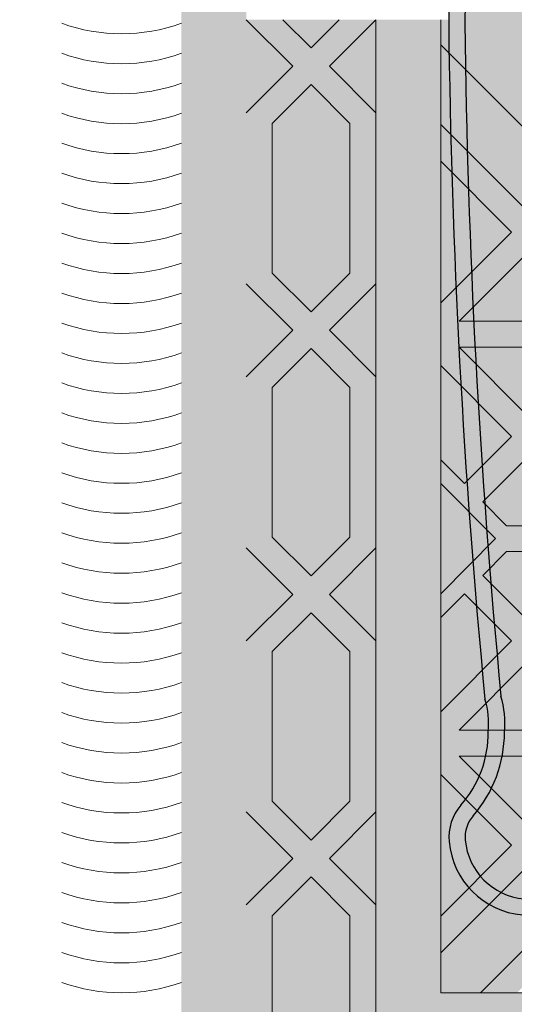
# Model space of a CAD drawing. Units: inches. Extents: x 844 to 2234, y 346 to 1084.
# Tile 9 of 93: x 1114.251 to 1119.118, y 686.542 to 696.22. Entities that reach past the tile are written whole.
import ezdxf

# ---------------------------------------------------------------- set-up
doc = ezdxf.new("R2010")
doc.units = ezdxf.units.IN
doc.header["$MEASUREMENT"] = 0
for name, color, linetype, lineweight in [('A-ANNO-DIMS', 2, 'Continuous', 18), ('furniture', 8, 'Continuous', 18), ('RA-AP-01$0$INT', 35, 'Continuous', 5)]:
    doc.layers.add(name, color=color, linetype=linetype, lineweight=lineweight)
doc.layers.add('RA-AP-01$0$FURN', color=3, linetype='Continuous')
doc.layers.add('RA-AP-01$0$WOOD', color=64, linetype='Continuous')
doc.styles.get("Standard").update_dxf_attribs({"font": 'arial.ttf'})
doc.dimstyles.get("Standard").update_dxf_attribs({"dimtxt": 6, "dimasz": 3, "dimexe": 0.18, "dimexo": 0.0625, "dimgap": 0.09, "dimtad": 0, "dimtih": 1, "dimtoh": 1, "dimdec": 1, "dimzin": 0, "dimdsep": 46, "dimlunit": 3, "dimtxsty": 'Standard', "dimblk": 'ARCHTICK', "dimcen": 0.09, "dimadec": 0, "dimazin": 0, "dimtfac": 1, "dimtdec": 1, "dimtofl": 0, "dimtmove": 0, "dimatfit": 3, "dimfxl": 1, "dimtolj": 1, "dimtzin": 0, "dimarcsym": 0})

# ---------------------------------------------------------------- blocks, each defined once
blk = doc.blocks.new('A$C18D01794')
at = {"layer": 'RA-AP-01$0$INT'}
h = blk.add_hatch(color=256, dxfattribs=at)
h.paths.add_polyline_path([(4.35521, -6.15671), (4.35521, -8.05671), (5.45521, -8.05671), (5.45521, -6.15671)])
h.paths.add_polyline_path([(4.40521, -8.00671), (4.40521, -6.20671), (5.40521, -6.20671), (5.40521, -8.00671)], flags=16)
h = blk.add_hatch(color=256, dxfattribs=at)
h.paths.add_polyline_path([(4.46935, -7.07085), (4.50521, -7.035), (4.50521, -7.10671)])
h.paths.add_polyline_path([(4.45521, -7.085), (4.47692, -7.10671), (4.43349, -7.10671)])
h.paths.add_polyline_path([(4.40521, -7.035), (4.44106, -7.07085), (4.40521, -7.10671)])
h.paths.add_polyline_path([(4.42521, -6.91146), (4.45521, -6.88146), (4.48521, -6.91146), (4.48521, -7.02671), (4.45521, -7.05671), (4.42521, -7.02671)])
h.paths.add_polyline_path([(4.50521, -6.83146), (4.50521, -6.90318), (4.46935, -6.86732)])
h.paths.add_polyline_path([(4.42521, -6.70793), (4.45521, -6.67793), (4.48521, -6.70793), (4.48521, -6.82318), (4.45521, -6.85318), (4.42521, -6.82318)])
h.paths.add_polyline_path([(4.42521, -6.50439), (4.45521, -6.47439), (4.48521, -6.50439), (4.48521, -6.61964), (4.45521, -6.64964), (4.42521, -6.61964)])
h.paths.add_polyline_path([(4.46935, -6.66378), (4.50521, -6.62793), (4.50521, -6.69964)])
h.paths.add_polyline_path([(4.40521, -6.62793), (4.44106, -6.66378), (4.40521, -6.69964)])
h.paths.add_polyline_path([(4.40521, -6.42439), (4.44106, -6.46025), (4.40521, -6.49611)])
h.paths.add_polyline_path([(4.46935, -6.46025), (4.50521, -6.42439), (4.50521, -6.49611)])
h.paths.add_polyline_path([(4.42521, -6.30085), (4.45521, -6.27085), (4.48521, -6.30085), (4.48521, -6.41611), (4.45521, -6.44611), (4.42521, -6.41611)])
h.paths.add_polyline_path([(4.42521, -6.22671), (4.47106, -6.22671), (4.42521, -6.27257)])
h.paths.add_polyline_path([(4.49935, -6.22671), (4.63606, -6.22671), (4.66606, -6.25671), (4.63606, -6.28671), (4.49935, -6.28671), (4.46935, -6.25671)])
h.paths.add_polyline_path([(4.68021, -6.27085), (4.71606, -6.30671), (4.64435, -6.30671)])
h.paths.add_polyline_path([(4.64435, -6.20671), (4.71606, -6.20671), (4.68021, -6.24257)])
h.paths.add_polyline_path([(4.72435, -6.22671), (4.86106, -6.22671), (4.89106, -6.25671), (4.86106, -6.28671), (4.72435, -6.28671), (4.69435, -6.25671)])
h.paths.add_polyline_path([(4.90521, -6.27085), (4.94106, -6.30671), (4.86935, -6.30671)])
h.paths.add_polyline_path([(4.86935, -6.20671), (4.94106, -6.20671), (4.90521, -6.24257)])
h.paths.add_polyline_path([(4.94935, -6.22671), (5.08606, -6.22671), (5.11606, -6.25671), (5.08606, -6.28671), (4.94935, -6.28671), (4.91935, -6.25671)])
h.paths.add_polyline_path([(5.13021, -6.27085), (5.16606, -6.30671), (5.09435, -6.30671)])
h.paths.add_polyline_path([(5.09435, -6.20671), (5.16606, -6.20671), (5.13021, -6.24257)])
h.paths.add_polyline_path([(5.17435, -6.22671), (5.31106, -6.22671), (5.34106, -6.25671), (5.31106, -6.28671), (5.17435, -6.28671), (5.14435, -6.25671)])
h.paths.add_polyline_path([(5.32521, -6.30085), (5.35521, -6.27085), (5.38521, -6.30085), (5.38521, -6.41611), (5.35521, -6.44611), (5.32521, -6.41611)])
h.paths.add_polyline_path([(5.33935, -6.22671), (5.38521, -6.22671), (5.38521, -6.27257)])
h.paths.add_polyline_path([(5.32521, -6.50439), (5.35521, -6.47439), (5.38521, -6.50439), (5.38521, -6.61964), (5.35521, -6.64964), (5.32521, -6.61964)])
h.paths.add_polyline_path([(5.30521, -6.42439), (5.34106, -6.46025), (5.30521, -6.49611)])
h.paths.add_polyline_path([(5.36935, -6.46025), (5.40521, -6.42439), (5.40521, -6.49611)])
h.paths.add_polyline_path([(5.40521, -6.62793), (5.40521, -6.69964), (5.36935, -6.66378)])
h.paths.add_polyline_path([(5.30521, -6.62793), (5.34106, -6.66378), (5.30521, -6.69964)])
h.paths.add_polyline_path([(5.32521, -6.70793), (5.35521, -6.67793), (5.38521, -6.70793), (5.38521, -6.82318), (5.35521, -6.85318), (5.32521, -6.82318)])
h.paths.add_polyline_path([(5.30521, -6.83146), (5.34106, -6.86732), (5.30521, -6.90318)])
h.paths.add_polyline_path([(5.32521, -6.91146), (5.35521, -6.88146), (5.38521, -6.91146), (5.38521, -7.02671), (5.35521, -7.05671), (5.32521, -7.02671)])
h.paths.add_polyline_path([(5.40458, -6.83209, 0.001218), (5.40521, -6.83231), (5.40521, -6.90318), (5.36935, -6.86732)])
h.paths.add_polyline_path([(5.36935, -7.07085), (5.40521, -7.035), (5.40521, -7.10671)])
h.paths.add_polyline_path([(5.35521, -7.085), (5.37692, -7.10671), (5.33349, -7.10671)])
h.paths.add_polyline_path([(5.30521, -7.035), (5.34106, -7.07085), (5.30521, -7.10671)])
h = blk.add_hatch(color=256, dxfattribs=at)
h.paths.add_polyline_path([(4.50521, -6.62793), (4.46935, -6.66378), (4.50521, -6.69964), (4.50521, -6.83146), (4.46935, -6.86732), (4.50521, -6.90318), (4.50521, -7.035), (4.46935, -7.07085), (4.50521, -7.10671), (4.47692, -7.10671), (4.45521, -7.085), (4.43349, -7.10671), (4.40521, -7.10671), (4.44106, -7.07085), (4.40521, -7.035), (4.40521, -6.90318), (4.44106, -6.86732), (4.40521, -6.83146), (4.40521, -6.69964), (4.44106, -6.66378), (4.40521, -6.62793), (4.40521, -6.49611), (4.44106, -6.46025), (4.40521, -6.42439), (4.40521, -6.20671), (4.64435, -6.20671), (4.68021, -6.24257), (4.71606, -6.20671), (4.86935, -6.20671), (4.90521, -6.24257), (4.94106, -6.20671), (5.09435, -6.20671), (5.13021, -6.24257), (5.16606, -6.20671), (5.40521, -6.20671), (5.40521, -6.42439), (5.36935, -6.46025), (5.40521, -6.49611), (5.40521, -6.62793), (5.36935, -6.66378), (5.40521, -6.69964), (5.40521, -6.83146), (5.36935, -6.86732), (5.40521, -6.90318), (5.40521, -7.035), (5.36935, -7.07085), (5.40521, -7.10671), (5.37692, -7.10671), (5.35521, -7.085), (5.33349, -7.10671), (5.30521, -7.10671), (5.34106, -7.07085), (5.30521, -7.035), (5.30521, -6.90318), (5.34106, -6.86732), (5.30521, -6.83146), (5.30521, -6.69964), (5.34106, -6.66378), (5.30521, -6.62793), (5.30521, -6.49611), (5.34106, -6.46025), (5.30521, -6.42439), (5.30521, -6.30671), (5.16606, -6.30671), (5.13021, -6.27085), (5.09435, -6.30671), (4.94106, -6.30671), (4.90521, -6.27085), (4.86935, -6.30671), (4.71606, -6.30671), (4.68021, -6.27085), (4.64435, -6.30671), (4.50521, -6.30671), (4.50521, -6.42439), (4.46935, -6.46025), (4.50521, -6.49611)])
h.paths.add_polyline_path([(4.48521, -6.50439), (4.45521, -6.47439), (4.42521, -6.50439), (4.42521, -6.61964), (4.45521, -6.64964), (4.48521, -6.61964)], flags=16)
h.paths.add_polyline_path([(4.45521, -6.44611), (4.48521, -6.41611), (4.48521, -6.30085), (4.45521, -6.27085), (4.42521, -6.30085), (4.42521, -6.41611)], flags=16)
h.paths.add_polyline_path([(4.45521, -6.67793), (4.42521, -6.70793), (4.42521, -6.82318), (4.45521, -6.85318), (4.48521, -6.82318), (4.48521, -6.70793)], flags=16)
h.paths.add_polyline_path([(4.49935, -6.28671), (4.63606, -6.28671), (4.66606, -6.25671), (4.63606, -6.22671), (4.49935, -6.22671), (4.46935, -6.25671)], flags=16)
h.paths.add_polyline_path([(4.42521, -6.27257), (4.47106, -6.22671), (4.42521, -6.22671)], flags=16)
h.paths.add_polyline_path([(4.45521, -6.88146), (4.42521, -6.91146), (4.42521, -7.02671), (4.45521, -7.05671), (4.48521, -7.02671), (4.48521, -6.91146)], flags=16)
h.paths.add_polyline_path([(4.72435, -6.28671), (4.86106, -6.28671), (4.89106, -6.25671), (4.86106, -6.22671), (4.72435, -6.22671), (4.69435, -6.25671)], flags=16)
h.paths.add_polyline_path([(4.91935, -6.25671), (4.94935, -6.28671), (5.08606, -6.28671), (5.11606, -6.25671), (5.08606, -6.22671), (4.94935, -6.22671)], flags=16)
h.paths.add_polyline_path([(5.14435, -6.25671), (5.17435, -6.28671), (5.31106, -6.28671), (5.34106, -6.25671), (5.31106, -6.22671), (5.17435, -6.22671)], flags=16)
h.paths.add_polyline_path([(5.32521, -6.61964), (5.35521, -6.64964), (5.38521, -6.61964), (5.38521, -6.50439), (5.35521, -6.47439), (5.32521, -6.50439)], flags=16)
h.paths.add_polyline_path([(5.32521, -6.41611), (5.35521, -6.44611), (5.38521, -6.41611), (5.38521, -6.30085), (5.35521, -6.27085), (5.32521, -6.30085)], flags=16)
h.paths.add_polyline_path([(5.32521, -6.70793), (5.32521, -6.82318), (5.35521, -6.85318), (5.38521, -6.82318), (5.38521, -6.70793), (5.35521, -6.67793)], flags=16)
h.paths.add_polyline_path([(5.32521, -6.91146), (5.32521, -7.02671), (5.35521, -7.05671), (5.38521, -7.02671), (5.38521, -6.91146), (5.35521, -6.88146)], flags=16)
h.paths.add_polyline_path([(5.33935, -6.22671), (5.38521, -6.27257), (5.38521, -6.22671)], flags=16)
for points in [[(4.50521, -6.30671), (5.30521, -6.30671), (5.30521, -7.10671), (5.25521, -7.10671), (5.25521, -6.35671), (4.55521, -6.35671), (4.55521, -7.10671), (4.50521, -7.10671)], [(4.40521, -6.90318), (4.44106, -6.86732), (4.40521, -6.83146)]]:
    blk.add_hatch(color=256, dxfattribs=at).paths.add_polyline_path(points)
h = blk.add_hatch(color=256, dxfattribs=at)
h.paths.add_polyline_path([(4.58592, -6.35671), (4.55521, -6.35671), (4.55521, -6.38742), (4.8745, -6.70671), (4.90521, -6.676)])
h.paths.add_polyline_path([(5.25521, -6.38742), (5.25521, -6.35671), (5.2245, -6.35671), (4.90521, -6.676), (4.93592, -6.70671)])
h.paths.add_polyline_path([(4.93592, -6.70671), (4.90521, -6.73742), (5.25521, -7.08742), (5.25521, -7.026)])
h.paths.add_polyline_path([(4.55521, -7.026), (4.55521, -7.08742), (4.90521, -6.73742), (4.8745, -6.70671)])
h = blk.add_hatch(color=256, dxfattribs=at)
h.paths.add_polyline_path([(4.58592, -6.35671), (4.6142, -6.35671), (4.66885, -6.41136), (4.72349, -6.35671), (4.77177, -6.35671), (4.82642, -6.41136), (4.86278, -6.375), (4.8445, -6.35671), (4.86278, -6.35671), (4.90521, -6.39914), (4.94763, -6.35671), (4.96592, -6.35671), (4.94763, -6.375), (4.98399, -6.41136), (5.03864, -6.35671), (5.08692, -6.35671), (5.14157, -6.41136), (5.19621, -6.35671), (5.2245, -6.35671), (4.90521, -6.676)])
h.paths.add_polyline_path([(4.89521, -6.63772), (4.89521, -6.52843), (4.84056, -6.58307)], flags=16)
h.paths.add_polyline_path([(4.91521, -6.63772), (4.96985, -6.58307), (4.91521, -6.52843)], flags=16)
h.paths.add_polyline_path([(4.82642, -6.56893), (4.88106, -6.51429), (4.77177, -6.51429)], flags=16)
h.paths.add_polyline_path([(4.98399, -6.56893), (5.03864, -6.51429), (4.92935, -6.51429)], flags=16)
h.paths.add_polyline_path([(4.88106, -6.49429), (4.82642, -6.43964), (4.77177, -6.49429)], flags=16)
h.paths.add_polyline_path([(4.92935, -6.49429), (5.03864, -6.49429), (4.98399, -6.43964)], flags=16)
h.paths.add_polyline_path([(4.89521, -6.48014), (4.89521, -6.40742), (4.87692, -6.38914), (4.84056, -6.4255)], flags=16)
h.paths.add_polyline_path([(4.91521, -6.48014), (4.96985, -6.4255), (4.93349, -6.38914), (4.91521, -6.40742)], flags=16)
h.paths.add_polyline_path([(4.75763, -6.48014), (4.81228, -6.4255), (4.75763, -6.37085)], flags=16)
h.paths.add_polyline_path([(4.73763, -6.48014), (4.73763, -6.37085), (4.68299, -6.4255)], flags=16)
h.paths.add_polyline_path([(5.05278, -6.48014), (5.05278, -6.37085), (4.99814, -6.4255)], flags=16)
h.paths.add_polyline_path([(5.07278, -6.48014), (5.12742, -6.4255), (5.07278, -6.37085)], flags=16)
h.paths.add_polyline_path([(4.93592, -6.70671), (5.25521, -6.38742), (5.25521, -6.41571), (5.20056, -6.47035), (5.25521, -6.525), (5.25521, -6.57328), (5.20056, -6.62793), (5.23692, -6.66429), (5.25521, -6.646), (5.25521, -6.66429), (5.21278, -6.70671), (5.25521, -6.74914), (5.25521, -6.76742), (5.23692, -6.74914), (5.20056, -6.7855), (5.25521, -6.84014), (5.25521, -6.88843), (5.20056, -6.94307), (5.25521, -6.99772), (5.25521, -7.026)])
h.paths.add_polyline_path([(5.04299, -6.7855), (5.09763, -6.84014), (5.09763, -6.73085)], flags=16)
h.paths.add_polyline_path([(5.02885, -6.77136), (5.08349, -6.71671), (4.9742, -6.71671)], flags=16)
h.paths.add_polyline_path([(5.11763, -6.84014), (5.17228, -6.7855), (5.11763, -6.73085)], flags=16)
h.paths.add_polyline_path([(5.08349, -6.69671), (5.02885, -6.64207), (4.9742, -6.69671)], flags=16)
h.paths.add_polyline_path([(5.13177, -6.85429), (5.18642, -6.79964), (5.24106, -6.85429)], flags=17)
h.paths.add_polyline_path([(5.13177, -6.71671), (5.18642, -6.77136), (5.22278, -6.735), (5.2045, -6.71671)], flags=16)
h.paths.add_polyline_path([(5.09763, -6.68257), (5.09763, -6.57328), (5.04299, -6.62793)], flags=16)
h.paths.add_polyline_path([(5.13177, -6.87429), (5.24106, -6.87429), (5.18642, -6.92893)], flags=17)
h.paths.add_polyline_path([(5.13177, -6.69671), (5.2045, -6.69671), (5.22278, -6.67843), (5.18642, -6.64207)], flags=16)
h.paths.add_polyline_path([(5.11763, -6.68257), (5.17228, -6.62793), (5.11763, -6.57328)], flags=16)
h.paths.add_polyline_path([(5.18642, -6.61378), (5.24106, -6.55914), (5.13177, -6.55914)], flags=16)
h.paths.add_polyline_path([(5.13177, -6.53914), (5.24106, -6.53914), (5.18642, -6.48449)], flags=16)
h.paths.add_polyline_path([(5.25521, -7.08742), (5.25521, -7.10671), (4.55521, -7.10671), (4.55521, -7.08742), (4.90521, -6.73742)])
h.paths.add_polyline_path([(4.98399, -6.84449), (4.92935, -6.89914), (5.03864, -6.89914)], flags=16)
h.paths.add_polyline_path([(4.96985, -6.83035), (4.91521, -6.77571), (4.91521, -6.885)], flags=16)
h.paths.add_polyline_path([(4.92935, -6.91914), (4.98399, -6.97378), (5.03864, -6.91914)], flags=16)
h.paths.add_polyline_path([(5.05278, -6.93328), (4.99814, -6.98793), (5.05278, -7.04257)], flags=16)
h.paths.add_polyline_path([(5.07278, -6.93328), (5.07278, -7.04257), (5.12742, -6.98793)], flags=16)
h.paths.add_polyline_path([(4.89521, -6.77571), (4.84056, -6.83035), (4.89521, -6.885)], flags=16)
h.paths.add_polyline_path([(4.91521, -6.93328), (4.91521, -7.006), (4.93349, -7.02429), (4.96985, -6.98793)], flags=16)
h.paths.add_polyline_path([(4.88106, -6.89914), (4.82642, -6.84449), (4.77177, -6.89914)], flags=16)
h.paths.add_polyline_path([(4.89521, -6.93328), (4.84056, -6.98793), (4.87692, -7.02429), (4.89521, -7.006)], flags=16)
h.paths.add_polyline_path([(4.98399, -7.00207), (4.94763, -7.03843), (4.96592, -7.05671), (5.03864, -7.05671)], flags=16)
h.paths.add_polyline_path([(4.88106, -6.91914), (4.77177, -6.91914), (4.82642, -6.97378)], flags=16)
h.paths.add_polyline_path([(4.90521, -7.01429), (4.86278, -7.05671), (4.94763, -7.05671)], flags=16)
h.paths.add_polyline_path([(5.14157, -7.00207), (5.08692, -7.05671), (5.19621, -7.05671)], flags=16)
h.paths.add_polyline_path([(4.82642, -7.00207), (4.77177, -7.05671), (4.8445, -7.05671), (4.86278, -7.03843)], flags=16)
h.paths.add_polyline_path([(4.81228, -6.98793), (4.75763, -6.93328), (4.75763, -7.04257)], flags=16)
h.paths.add_polyline_path([(4.73763, -6.93328), (4.68299, -6.98793), (4.73763, -7.04257)], flags=16)
h.paths.add_polyline_path([(4.72349, -7.05671), (4.66885, -7.00207), (4.6142, -7.05671)], flags=16)
h.paths.add_polyline_path([(4.59763, -6.70671), (4.55521, -6.66429), (4.55521, -6.646), (4.57349, -6.66429), (4.60985, -6.62793), (4.55521, -6.57328), (4.55521, -6.525), (4.60985, -6.47035), (4.55521, -6.41571), (4.55521, -6.38742), (4.8745, -6.70671), (4.55521, -7.026), (4.55521, -6.99772), (4.60985, -6.94307), (4.55521, -6.88843), (4.55521, -6.84014), (4.60985, -6.7855), (4.57349, -6.74914), (4.55521, -6.76742), (4.55521, -6.74914)])
h.paths.add_polyline_path([(4.71278, -6.73085), (4.71278, -6.84014), (4.76742, -6.7855)], flags=16)
h.paths.add_polyline_path([(4.72692, -6.71671), (4.78157, -6.77136), (4.83621, -6.71671)], flags=16)
h.paths.add_polyline_path([(4.69278, -6.73085), (4.63814, -6.7855), (4.69278, -6.84014)], flags=16)
h.paths.add_polyline_path([(4.72692, -6.69671), (4.83621, -6.69671), (4.78157, -6.64207)], flags=16)
h.paths.add_polyline_path([(4.67864, -6.71671), (4.60592, -6.71671), (4.58763, -6.735), (4.62399, -6.77136)], flags=16)
h.paths.add_polyline_path([(4.71278, -6.68257), (4.76742, -6.62793), (4.71278, -6.57328)], flags=16)
h.paths.add_polyline_path([(4.67864, -6.69671), (4.62399, -6.64207), (4.58763, -6.67843), (4.60592, -6.69671)], flags=16)
h.paths.add_polyline_path([(4.69278, -6.68257), (4.69278, -6.57328), (4.63814, -6.62793)], flags=16)
h.paths.add_polyline_path([(4.62399, -6.79964), (4.67864, -6.85429), (4.56935, -6.85429)], flags=17)
h.paths.add_polyline_path([(4.62399, -6.61378), (4.67864, -6.55914), (4.56935, -6.55914)], flags=16)
h.paths.add_polyline_path([(4.67864, -6.87429), (4.62399, -6.92893), (4.56935, -6.87429)], flags=17)
h.paths.add_polyline_path([(4.67864, -6.53914), (4.62399, -6.48449), (4.56935, -6.53914)], flags=16)
h = blk.add_hatch(color=256, dxfattribs=at)
h.paths.add_polyline_path([(4.78157, -6.77136), (4.83621, -6.71671), (4.72692, -6.71671)])
h.paths.add_polyline_path([(4.83621, -6.69671), (4.78157, -6.64207), (4.72692, -6.69671)])
h.paths.add_polyline_path([(4.76742, -6.62793), (4.71278, -6.57328), (4.71278, -6.68257)])
h.paths.add_polyline_path([(4.69278, -6.68257), (4.69278, -6.57328), (4.63814, -6.62793)])
h.paths.add_polyline_path([(4.67864, -6.69671), (4.62399, -6.64207), (4.58763, -6.67843), (4.60592, -6.69671)])
h.paths.add_polyline_path([(4.57349, -6.66429), (4.60985, -6.62793), (4.55521, -6.57328), (4.55521, -6.646)])
h.paths.add_polyline_path([(4.62399, -6.61378), (4.67864, -6.55914), (4.56935, -6.55914)])
h.paths.add_polyline_path([(4.67864, -6.53914), (4.62399, -6.48449), (4.56935, -6.53914)])
h.paths.add_polyline_path([(4.60985, -6.47035), (4.55521, -6.41571), (4.55521, -6.525)])
h.paths.add_polyline_path([(4.59763, -6.70671), (4.55521, -6.66429), (4.55521, -6.74914)])
h.paths.add_polyline_path([(4.67864, -6.71671), (4.60592, -6.71671), (4.58763, -6.735), (4.62399, -6.77136)])
h.paths.add_polyline_path([(4.69278, -6.84014), (4.69278, -6.73085), (4.63814, -6.7855)])
h.paths.add_polyline_path([(4.76742, -6.7855), (4.71278, -6.73085), (4.71278, -6.84014)])
h.paths.add_polyline_path([(4.67864, -6.85429), (4.62399, -6.79964), (4.56935, -6.85429)])
h.paths.add_polyline_path([(4.60985, -6.7855), (4.57349, -6.74914), (4.55521, -6.76742), (4.55521, -6.84014)])
h.paths.add_polyline_path([(4.62399, -6.92893), (4.67864, -6.87429), (4.56935, -6.87429)])
h.paths.add_polyline_path([(4.60985, -6.94307), (4.55521, -6.88843), (4.55521, -6.99772)])
for p, q in [((4.42521, -6.41611), (4.42521, -6.30085)), ((4.48521, -6.30085), (4.48521, -6.41611)), ((4.55521, -6.35671), (5.25521, -6.35671)), ((4.55521, -7.10671), (4.55521, -6.35671)), ((4.90521, -6.676), (4.58592, -6.35671)), ((4.8745, -6.70671), (4.55521, -6.38742)), ((4.45521, -6.44611), (4.42521, -6.41611)), ((4.45521, -6.44611), (4.48521, -6.41611)), ((4.55521, -6.41571), (4.60985, -6.47035)), ((4.44106, -6.46025), (4.40521, -6.42439)), ((4.46935, -6.46025), (4.50521, -6.42439)), ((4.40521, -6.49611), (4.44106, -6.46025)), ((4.50521, -6.49611), (4.46935, -6.46025)), ((4.55521, -6.525), (4.60985, -6.47035)), ((4.42521, -6.50439), (4.45521, -6.47439)), ((4.48521, -6.50439), (4.45521, -6.47439)), ((4.56935, -6.53914), (4.62399, -6.48449)), ((4.42521, -6.61964), (4.42521, -6.50439)), ((4.48521, -6.61964), (4.48521, -6.50439)), ((4.67864, -6.53914), (4.56935, -6.53914)), ((4.56935, -6.55914), (4.62399, -6.61378)), ((4.67864, -6.55914), (4.56935, -6.55914)), ((4.55521, -6.646), (4.55521, -6.57328)), ((4.55521, -6.57328), (4.60985, -6.62793)), ((4.42521, -6.61964), (4.45521, -6.64964)), ((4.48521, -6.61964), (4.45521, -6.64964)), ((4.40521, -6.62793), (4.44106, -6.66378)), ((4.50521, -6.62793), (4.46935, -6.66378)), ((4.60985, -6.62793), (4.57349, -6.66429)), ((4.55521, -6.646), (4.57349, -6.66429)), ((4.62399, -6.64207), (4.58763, -6.67843)), ((4.40521, -6.69964), (4.44106, -6.66378)), ((4.50521, -6.69964), (4.46935, -6.66378)), ((4.55521, -6.74914), (4.55521, -6.66429)), ((4.59763, -6.70671), (4.55521, -6.66429)), ((4.42521, -6.70793), (4.45521, -6.67793)), ((4.48521, -6.70793), (4.45521, -6.67793)), ((4.60592, -6.69671), (4.58763, -6.67843)), ((4.60592, -6.69671), (4.67864, -6.69671)), ((4.42521, -6.82318), (4.42521, -6.70793)), ((4.48521, -6.82318), (4.48521, -6.70793)), ((4.8745, -6.70671), (4.55521, -7.026)), ((4.59763, -6.70671), (4.55521, -6.74914)), ((4.60592, -6.71671), (4.58763, -6.735)), ((4.60592, -6.71671), (4.67864, -6.71671)), ((4.90521, -6.73742), (4.55521, -7.08742)), ((4.62399, -6.77136), (4.58763, -6.735)), ((4.57349, -6.74914), (4.55521, -6.76742)), ((4.55521, -6.76742), (4.57349, -6.74914)), ((4.60985, -6.7855), (4.57349, -6.74914)), ((4.55521, -6.76742), (4.55521, -6.84014)), ((4.55521, -6.84014), (4.60985, -6.7855)), ((4.56935, -6.85429), (4.62399, -6.79964)), ((4.42521, -6.82318), (4.45521, -6.85318)), ((4.48521, -6.82318), (4.45521, -6.85318)), ((4.40521, -6.83146), (4.44106, -6.86732)), ((4.50521, -6.83146), (4.46935, -6.86732)), ((4.67864, -6.85429), (4.56935, -6.85429)), ((4.40521, -6.90318), (4.44106, -6.86732)), ((4.50521, -6.90318), (4.46935, -6.86732)), ((4.56935, -6.87429), (4.62399, -6.92893)), ((4.67864, -6.87429), (4.56935, -6.87429)), ((4.42521, -6.91146), (4.45521, -6.88146)), ((4.48521, -6.91146), (4.45521, -6.88146)), ((4.55521, -6.88843), (4.60985, -6.94307)), ((4.55521, -6.88843), (4.55521, -6.99772)), ((4.42521, -6.91146), (4.42521, -7.02671)), ((4.48521, -6.91146), (4.48521, -7.02671)), ((4.55521, -6.99772), (4.60985, -6.94307)), ((4.42521, -7.02671), (4.45521, -7.05671)), ((4.48521, -7.02671), (4.45521, -7.05671)), ((4.40521, -7.035), (4.44106, -7.07085)), ((4.50521, -7.035), (4.46935, -7.07085)), ((4.44106, -7.07085), (4.40521, -7.10671)), ((4.46935, -7.07085), (4.50521, -7.10671)), ((4.45521, -7.085), (4.43349, -7.10671)), ((4.45521, -7.085), (4.47692, -7.10671))]:
    blk.add_line(p, q, dxfattribs=at)
blk.add_lwpolyline([(5.30521, -7.10671), (5.30521, -6.30671), (4.50521, -6.30671), (4.50521, -7.10671)], dxfattribs=at)
for centre in [(4.30901, -6.49306), (4.30901, -6.51616), (4.30901, -6.53926), (4.30901, -6.56236), (4.30901, -6.58546), (4.30901, -6.60856), (4.30901, -6.63166), (4.30901, -6.65476), (4.30901, -6.67786), (4.30901, -6.70096), (4.30901, -6.72406), (4.30901, -6.74716), (4.30901, -6.77026), (4.30901, -6.79336), (4.30901, -6.79336), (4.30901, -6.81646), (4.30901, -6.83956), (4.30901, -6.86266), (4.30901, -6.88576), (4.30901, -6.90886), (4.30901, -6.93196), (4.30901, -6.95506), (4.30901, -6.97816), (4.30901, -7.00126), (4.30901, -7.02436), (4.30901, -7.04746), (4.30901, -7.07056), (4.30901, -7.09366), (4.30901, -7.11676), (4.30901, -7.13986), (4.30901, -7.16296), (4.30901, -7.18606), (4.30901, -7.20916), (4.30901, -7.23226)]:
    blk.add_arc(centre, 0.13641, 70.20384, 109.79616, dxfattribs=at)
blk = doc.blocks.new('A$C32926AE1')
at = {"layer": 'RA-AP-01$0$WOOD'}
h = blk.add_hatch(color=256, dxfattribs=at)
h.dxf.hatch_style = 1
h.paths.add_polyline_path([(5.15743, 4.57348, -0.100949), (5.1554, 4.59337, -0.184266), (5.17225, 4.6388, 0.205661), (5.17956, 4.66132, 0.361434), (5.13435, 4.70652, 0.205661), (5.11183, 4.69921, -0.184266), (5.0664, 4.68237, -0.105531), (5.04566, 4.68467, 0.156764), (4.76389, 4.68467, -0.105531), (4.74314, 4.68237, -0.184266), (4.69771, 4.69921, 0.205661), (4.67519, 4.70652, 0.361434), (4.62998, 4.66132, 0.205661), (4.63729, 4.6388, -0.184266), (4.65414, 4.59337, -0.100949), (4.65211, 4.57348, 0.02141), (4.62975, 4.15671, 0.02141), (4.65211, 3.73994, -0.100949), (4.65414, 3.72006, -0.184266), (4.63729, 3.67463, 0.205661), (4.62998, 3.65211, 0.361434), (4.67519, 3.6069, 0.205661), (4.69771, 3.61421, -0.184266), (4.74314, 3.63106, -0.105531), (4.76389, 3.62875, 0.156764), (5.04566, 3.62875, -0.105531), (5.0664, 3.63106, -0.184266), (5.11183, 3.61421, 0.205661), (5.13435, 3.6069, 0.361434), (5.17956, 3.65211, 0.205661), (5.17225, 3.67463, -0.184266), (5.1554, 3.72006, -0.100949), (5.15743, 3.73994, 0.02141), (5.17979, 4.15671, 0.02141)])
h.paths.add_polyline_path([(4.63975, 4.15671, 0.021354), (4.66197, 3.74189, -0.094076), (4.66414, 3.71961, -0.182482), (4.64481, 3.66804, 0.205661), (4.63994, 3.65302, 0.361434), (4.67611, 3.61686, 0.205661), (4.69112, 3.62173, -0.182482), (4.7427, 3.64106, -0.102989), (4.76699, 3.63826, 0.156709), (5.04255, 3.63826, -0.102989), (5.06685, 3.64106, -0.182482), (5.11842, 3.62173, 0.205661), (5.13344, 3.61686, 0.361434), (5.1696, 3.65302, 0.205661), (5.16473, 3.66804, -0.182482), (5.1454, 3.71961, -0.094076), (5.14757, 3.74189, 0.021354), (5.16979, 4.15671, 0.021354), (5.14757, 4.57154, -0.094076), (5.1454, 4.59381, -0.182482), (5.16473, 4.64539, 0.205661), (5.1696, 4.6604, 0.361434), (5.13344, 4.69657, 0.205661), (5.11842, 4.69169, -0.182482), (5.06685, 4.67236, -0.102989), (5.04255, 4.67517, 0.156709), (4.76699, 4.67517, -0.102989), (4.7427, 4.67236, -0.182482), (4.69112, 4.69169, 0.205661), (4.67611, 4.69657, 0.361434), (4.63994, 4.6604, 0.205661), (4.64481, 4.64539, -0.182482), (4.66414, 4.59381, -0.094076), (4.66197, 4.57154, 0.021354)], flags=16)
h.paths.add_polyline_path([(5.12979, 4.43217, -0.014166), (5.13015, 4.15693, -0.014166), (5.12979, 3.88169, -0.078525), (5.1098, 3.75514, 0.094597), (5.10541, 3.7179, 0.104317), (5.11607, 3.67039, 0.104317), (5.06856, 3.68105, 0.094597), (5.03132, 3.67666, -0.158024), (4.77823, 3.67666, 0.094597), (4.74098, 3.68105, 0.104317), (4.69347, 3.67039, 0.104317), (4.70413, 3.7179, 0.094597), (4.69975, 3.75514, -0.078525), (4.67975, 3.88169, -0.014166), (4.67939, 4.15693, -0.014166), (4.67975, 4.43217, -0.078525), (4.69975, 4.55871, 0.094597), (4.70413, 4.59596, 0.104317), (4.69347, 4.64347, 0.104317), (4.74098, 4.6328, 0.094597), (4.77823, 4.63719, -0.158024), (5.03132, 4.63719, 0.094597), (5.06856, 4.6328, 0.104317), (5.11607, 4.64347, 0.104317), (5.10541, 4.59596, 0.094597), (5.1098, 4.55871, -0.078525)], flags=0)
h.paths.add_polyline_path([(5.11979, 4.43226, -0.0142), (5.12016, 4.15693, -0.0142), (5.11979, 3.8816, -0.078489), (5.10027, 3.75819, 0.094014), (5.09541, 3.71748, 0.060627), (5.09962, 3.68684, 0.060627), (5.06898, 3.69105, 0.094014), (5.02827, 3.68619, -0.158071), (4.78127, 3.68619, 0.094014), (4.74056, 3.69105, 0.060627), (4.70993, 3.68684, 0.060627), (4.71413, 3.71748, 0.094014), (4.70927, 3.75819, -0.078489), (4.68975, 3.8816, -0.0142), (4.68939, 4.15693, -0.0142), (4.68975, 4.43226, -0.078489), (4.70927, 4.55566, 0.094014), (4.71413, 4.59638, 0.060627), (4.70993, 4.62701, 0.060627), (4.74056, 4.62281, 0.094014), (4.78127, 4.62767, -0.158071), (5.02827, 4.62767, 0.094014), (5.06898, 4.62281, 0.060627), (5.09962, 4.62701, 0.060627), (5.09541, 4.59638, 0.094014), (5.10027, 4.55566, -0.078489)], flags=0)
h.paths.add_polyline_path([(5.06979, 4.43022, -0.014242), (5.07017, 4.15693, -0.014242), (5.06979, 3.88364, -0.080061), (5.05266, 3.77346, 0.052642), (5.04591, 3.74055, 0.052642), (5.013, 3.7338, -0.158303), (4.79655, 3.7338, 0.052642), (4.76363, 3.74055, 0.052642), (4.75688, 3.77346, -0.080061), (4.73975, 3.88364, -0.014242), (4.73937, 4.15693, -0.014242), (4.73975, 4.43022, -0.080061), (4.75688, 4.54039, 0.052642), (4.76363, 4.5733, 0.052642), (4.79655, 4.58006, -0.158303), (5.013, 4.58006, 0.052642), (5.04591, 4.5733, 0.052642), (5.05266, 4.54039, -0.080061)], flags=0)
h.paths.add_polyline_path([(5.04979, 4.43038, -0.01431), (5.05018, 4.15693, -0.01431), (5.04979, 3.88347, -0.080069), (5.03362, 3.77958, 0.030626), (5.02824, 3.75822, 0.030626), (5.00688, 3.75284, -0.158398), (4.80266, 3.75284, 0.030626), (4.7813, 3.75822, 0.030626), (4.77592, 3.77958, -0.080069), (4.75975, 3.88347, -0.01431), (4.75936, 4.15693, -0.01431), (4.75975, 4.43038, -0.080069), (4.77592, 4.53427, 0.030626), (4.7813, 4.55564, 0.030626), (4.80266, 4.56102, -0.158398), (5.00688, 4.56102, 0.030626), (5.02824, 4.55564, 0.030626), (5.03362, 4.53427, -0.080069)], flags=0)
h.paths.add_polyline_path([(4.99977, 4.42817, -0.014344), (5.0002, 4.15693, -0.014344), (4.99977, 3.88568, -0.078464), (4.98736, 3.7991, -0.150605), (4.82219, 3.7991, -0.078464), (4.80978, 3.88568, -0.014344), (4.80934, 4.15693, -0.014344), (4.80978, 4.42817, -0.078464), (4.82219, 4.51475, -0.150605), (4.98736, 4.51475, -0.078464)], flags=0)
h.paths.add_polyline_path([(4.97976, 4.42764, -0.014377), (4.98021, 4.15693, -0.014377), (4.97976, 3.88621, -0.068924), (4.97118, 3.81528, -0.129665), (4.83836, 3.81528, -0.068924), (4.82979, 3.88621, -0.014377), (4.82934, 4.15693, -0.014377), (4.82979, 4.42764, -0.068924), (4.83836, 4.49858, -0.129665), (4.97118, 4.49858, -0.068924)], flags=0)
h = blk.add_hatch(color=256, dxfattribs=at)
h.dxf.hatch_style = 1
h.paths.add_polyline_path([(5.1454, 4.59381, -0.182482), (5.16473, 4.64539, 0.205661), (5.1696, 4.6604, 0.361434), (5.13344, 4.69657, 0.205661), (5.11842, 4.69169, -0.182482), (5.06685, 4.67236, -0.102989), (5.04255, 4.67517, 0.156709), (4.76699, 4.67517, -0.102989), (4.7427, 4.67236, -0.182482), (4.69112, 4.69169, 0.205661), (4.67611, 4.69657, 0.361434), (4.63994, 4.6604, 0.205661), (4.64481, 4.64539, -0.182482), (4.66414, 4.59381, -0.094076), (4.66197, 4.57154, 0.021354), (4.63975, 4.15671, 0.021354), (4.66197, 3.74189, -0.094076), (4.66414, 3.71961, -0.182482), (4.64481, 3.66804, 0.205661), (4.63994, 3.65302, 0.361434), (4.67611, 3.61686, 0.205661), (4.69112, 3.62173, -0.182482), (4.7427, 3.64106, -0.102989), (4.76699, 3.63826, 0.156709), (5.04255, 3.63826, -0.102989), (5.06685, 3.64106, -0.182482), (5.11842, 3.62173, 0.205661), (5.13344, 3.61686, 0.361434), (5.1696, 3.65302, 0.205661), (5.16473, 3.66804, -0.182482), (5.1454, 3.71961, -0.094076), (5.14757, 3.74189, 0.021354), (5.16979, 4.15671, 0.021354), (5.14757, 4.57154, -0.094076)])
h.paths.add_polyline_path([(5.1098, 4.55871, -0.078525), (5.12979, 4.43217, -0.014166), (5.13015, 4.15693, -0.014166), (5.12979, 3.88169, -0.078525), (5.1098, 3.75514, 0.094597), (5.10541, 3.7179, 0.104317), (5.11607, 3.67039, 0.104317), (5.06856, 3.68105, 0.094597), (5.03132, 3.67666, -0.158024), (4.77823, 3.67666, 0.094597), (4.74098, 3.68105, 0.104317), (4.69347, 3.67039, 0.104317), (4.70413, 3.7179, 0.094597), (4.69975, 3.75514, -0.078525), (4.67975, 3.88169, -0.014166), (4.67939, 4.15693, -0.014166), (4.67975, 4.43217, -0.078525), (4.69975, 4.55871, 0.094597), (4.70413, 4.59596, 0.104317), (4.69347, 4.64347, 0.104317), (4.74098, 4.6328, 0.094597), (4.77823, 4.63719, -0.158024), (5.03132, 4.63719, 0.094597), (5.06856, 4.6328, 0.104317), (5.11607, 4.64347, 0.104317), (5.10541, 4.59596, 0.094597)], flags=16)
h.paths.add_polyline_path([(5.10027, 4.55566, -0.078489), (5.11979, 4.43226, -0.0142), (5.12016, 4.15693, -0.0142), (5.11979, 3.8816, -0.078489), (5.10027, 3.75819, 0.094014), (5.09541, 3.71748, 0.060627), (5.09962, 3.68684, 0.060627), (5.06898, 3.69105, 0.094014), (5.02827, 3.68619, -0.158071), (4.78127, 3.68619, 0.094014), (4.74056, 3.69105, 0.060627), (4.70993, 3.68684, 0.060627), (4.71413, 3.71748, 0.094014), (4.70927, 3.75819, -0.078489), (4.68975, 3.8816, -0.0142), (4.68939, 4.15693, -0.0142), (4.68975, 4.43226, -0.078489), (4.70927, 4.55566, 0.094014), (4.71413, 4.59638, 0.060627), (4.70993, 4.62701, 0.060627), (4.74056, 4.62281, 0.094014), (4.78127, 4.62767, -0.158071), (5.02827, 4.62767, 0.094014), (5.06898, 4.62281, 0.060627), (5.09962, 4.62701, 0.060627), (5.09541, 4.59638, 0.094014)], flags=0)
h.paths.add_polyline_path([(5.04591, 4.5733, 0.052642), (5.05266, 4.54039, -0.080061), (5.06979, 4.43022, -0.014242), (5.07017, 4.15693, -0.014242), (5.06979, 3.88364, -0.080061), (5.05266, 3.77346, 0.052642), (5.04591, 3.74055, 0.052642), (5.013, 3.7338, -0.158303), (4.79655, 3.7338, 0.052642), (4.76363, 3.74055, 0.052642), (4.75688, 3.77346, -0.080061), (4.73975, 3.88364, -0.014242), (4.73937, 4.15693, -0.014242), (4.73975, 4.43022, -0.080061), (4.75688, 4.54039, 0.052642), (4.76363, 4.5733, 0.052642), (4.79655, 4.58006, -0.158303), (5.013, 4.58006, 0.052642)], flags=0)
h.paths.add_polyline_path([(5.02824, 4.55564, 0.030626), (5.03362, 4.53427, -0.080069), (5.04979, 4.43038, -0.01431), (5.05018, 4.15693, -0.01431), (5.04979, 3.88347, -0.080069), (5.03362, 3.77958, 0.030626), (5.02824, 3.75822, 0.030626), (5.00688, 3.75284, -0.158398), (4.80266, 3.75284, 0.030626), (4.7813, 3.75822, 0.030626), (4.77592, 3.77958, -0.080069), (4.75975, 3.88347, -0.01431), (4.75936, 4.15693, -0.01431), (4.75975, 4.43038, -0.080069), (4.77592, 4.53427, 0.030626), (4.7813, 4.55564, 0.030626), (4.80266, 4.56102, -0.158398), (5.00688, 4.56102, 0.030626)], flags=0)
h.paths.add_polyline_path([(4.98736, 4.51475, -0.078464), (4.99977, 4.42817, -0.014344), (5.0002, 4.15693, -0.014344), (4.99977, 3.88568, -0.078464), (4.98736, 3.7991, -0.150605), (4.82219, 3.7991, -0.078464), (4.80978, 3.88568, -0.014344), (4.80934, 4.15693, -0.014344), (4.80978, 4.42817, -0.078464), (4.82219, 4.51475, -0.150605)], flags=0)
h.paths.add_polyline_path([(4.97118, 4.49858, -0.068924), (4.97976, 4.42764, -0.014377), (4.98021, 4.15693, -0.014377), (4.97976, 3.88621, -0.068924), (4.97118, 3.81528, -0.129665), (4.83836, 3.81528, -0.068924), (4.82979, 3.88621, -0.014377), (4.82934, 4.15693, -0.014377), (4.82979, 4.42764, -0.068924), (4.83836, 4.49858, -0.129665)], flags=0)
for centre, radius, start, end in [((9.50522, 4.10408), 4.87575, 174.47541, 179.3815), ((9.50522, 4.10408), 4.86575, 174.48704, 179.3815), ((9.50522, 4.20934), 4.87575, 180.6185, 185.52459), ((9.50522, 4.20934), 4.86575, 180.6185, 185.51296), ((4.60439, 3.72503), 0.06, 354.82381, 16.32113), ((4.60439, 3.72503), 0.05, 354.29793, 17.35568), ((4.58617, 3.71943), 0.06797, 318.77105, 0.53331), ((4.58617, 3.71943), 0.07797, 318.77105, 0.13765), ((4.65986, 3.65486), 0.03, 138.77105, 185.25688), ((4.65986, 3.65486), 0.02, 138.77105, 185.25688), ((4.67977, 3.65669), 0.05, 185.25688, 264.74312), ((4.67977, 3.65669), 0.04, 185.25688, 264.74312)]:
    blk.add_arc(centre, radius, start, end, dxfattribs=at)
blk = doc.blocks.new('A$C5D2F253E')
at = {"layer": 'RA-AP-01$0$FURN', "xscale": -0.7999999999883585, "yscale": 0.7999999999883585, "zscale": 0.8, "rotation": 90}
blk.add_blockref('A$C18D01794', (-5.68776, 4.75792), dxfattribs=at)
at = {"layer": 'RA-AP-01$0$WOOD', "rotation": 270}
blk.add_blockref('A$C32926AE1', (-4.16134, 5.73853), dxfattribs=at)
blk = doc.blocks.new('_ArchTick')
at = {"color": 0, "linetype": 'ByBlock', "const_width": 0.15}
blk.add_lwpolyline([(-0.5, -0.5), (0.5, 0.5)], dxfattribs=at)
blk = doc.blocks.new('*D144')
at = {"layer": 'A-ANNO-DIMS', "color": 0, "lineweight": -2, "transparency": 16777216}
for p, q in [((1096.6159, 439.3733), (1096.6159, 1074.7433)), ((1143.1159, 492.3733), (1143.1159, 1074.7433)), ((1096.6159, 1074.5633), (1102.482, 1074.5633)), ((1143.1159, 1074.5633), (1137.2499, 1074.5633))]:
    blk.add_line(p, q, dxfattribs=at)
at = {"layer": 'Defpoints', "color": 0, "transparency": 16777216}
for p in [(1143.1159, 1074.5633), (1143.1159, 492.3108), (1096.6159, 439.3108)]:
    blk.add_point(p, dxfattribs=at)
at = {"layer": 'A-ANNO-DIMS', "color": 0, "lineweight": -2, "transparency": 16777216, "xscale": 3, "yscale": 3, "zscale": 3, "rotation": 180}
blk.add_blockref('_ArchTick', (1096.6159, 1074.5633), dxfattribs=at)
at = {"layer": 'A-ANNO-DIMS', "color": 0, "lineweight": -2, "transparency": 16777216, "xscale": 3, "yscale": 3, "zscale": 3}
blk.add_blockref('_ArchTick', (1143.1159, 1074.5633), dxfattribs=at)
at = {"layer": 'A-ANNO-DIMS', "color": 0, "transparency": 16777216, "insert": (1119.8659, 1074.5633), "char_height": 6, "attachment_point": 5}
blk.add_mtext('\\A1;3\'-10 1/2"', dxfattribs=at)

msp = doc.modelspace()

# ---------------------------------------------------------------- block references
at = {"layer": 'furniture', "xscale": 15.94108302203742, "yscale": 15.94108302203742, "zscale": 15.94108302203742, "rotation": 90}
msp.add_blockref('A$C5D2F253E', (1136.1478, 696.2585), dxfattribs=at)

# ---------------------------------------------------------------- dimensions: what is measured, and where the dimension line sits
at = {"layer": 'A-ANNO-DIMS'}
dim = msp.add_linear_dim(base=(1143.1159, 1074.5633), p1=(1096.6159, 439.3108), p2=(1143.1159, 492.3108), dimstyle='Standard', override={"dimdec": 1, "dimlfac": 1, "dimrnd": 0, "dimzin": 1, "dimdsep": 46, "dimlunit": 4, "dimfrac": 2}, dxfattribs=at)
dim.commit()
dim.dimension.update_dxf_attribs({"geometry": '*D144', "text_midpoint": (1119.8659, 1074.5633)})

doc.saveas('drawing.dxf')
